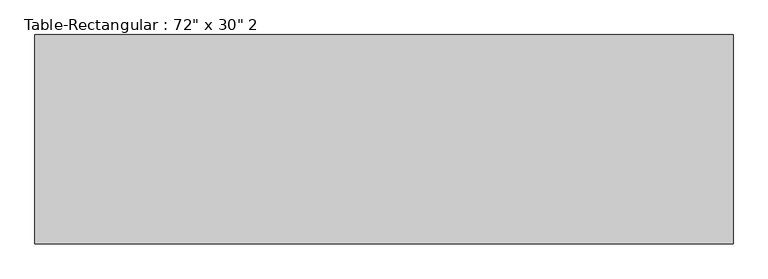
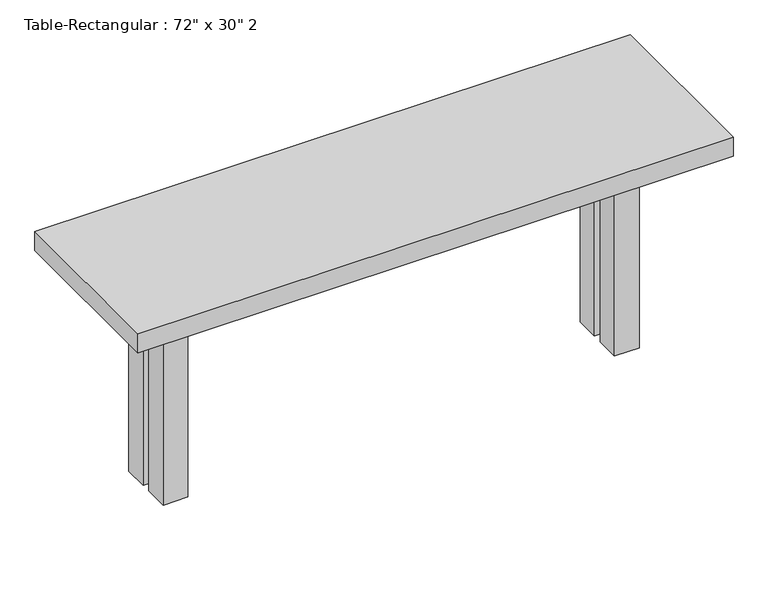
"""IFC4 building model written with IfcOpenShell, lengths in millimetres: furniture geometry."""

from ifc_helpers import new_model, si_unit, frame, origin, origin_with_axes, place, context, project, spatial, polyline, outline, extrude, source, transform, mapped, element, save


def furniture_87306a90(model_context):
    return source(origin(), model_context, "Body", "SweptSolid", [
        extrude(outline(polyline([(546.1, 38.1), (546.1, 12.7), (-546.1, 12.7), (-546.1, 38.1), (546.1, 38.1)])), frame((0.0, 0.0, 457.2), z_axis=(0.0, 0.0, 1.0), x_axis=(1.0, 0.0, 0.0)), (0.0, 0.0, 1.0), 101.6),
        extrude(outline(polyline([(546.1, -38.1), (-546.1, -38.1), (-546.1, -12.7), (546.1, -12.7), (546.1, -38.1)])), frame((0.0, 0.0, 457.2), z_axis=(0.0, 0.0, 1.0), x_axis=(1.0, 0.0, 0.0)), (0.0, 0.0, 1.0), 101.6),
        extrude(outline(polyline([(-558.8, -12.7), (-584.2, -12.7), (-584.2, 12.7), (-558.8, 12.7), (-558.8, -12.7)])), frame((0.0, 0.0, 457.2), z_axis=(0.0, 0.0, 1.0), x_axis=(1.0, 0.0, 0.0)), (0.0, 0.0, 1.0), 101.6),
        extrude(outline(polyline([(558.8, -12.7), (558.8, 12.7), (584.2, 12.7), (584.2, -12.7), (558.8, -12.7)])), frame((0.0, 0.0, 457.2), z_axis=(0.0, 0.0, 1.0), x_axis=(1.0, 0.0, 0.0)), (0.0, 0.0, 1.0), 101.6),
        extrude(outline(polyline([(762.0, 228.6), (762.0, -228.6), (-762.0, -228.6), (-762.0, 228.6), (762.0, 228.6)])), frame((0.0, 0.0, 558.8), z_axis=(0.0, 0.0, 1.0), x_axis=(1.0, 0.0, 0.0)), (0.0, 0.0, 1.0), 50.8),
        extrude(outline(polyline([(-546.1, 76.2), (-546.1, 12.7), (-609.6, 12.7), (-609.6, 76.2), (-546.1, 76.2)])), origin_with_axes(), (0.0, 0.0, 1.0), 558.8),
        extrude(outline(polyline([(546.1, 76.2), (609.6, 76.2), (609.6, 12.7), (546.1, 12.7), (546.1, 76.2)])), origin_with_axes(), (0.0, 0.0, 1.0), 558.8),
        extrude(outline(polyline([(-546.1, -76.2), (-609.6, -76.2), (-609.6, -12.7), (-546.1, -12.7), (-546.1, -76.2)])), origin_with_axes(), (0.0, 0.0, 1.0), 558.8),
        extrude(outline(polyline([(546.1, -76.2), (546.1, -12.7), (609.6, -12.7), (609.6, -76.2), (546.1, -76.2)])), origin_with_axes(), (0.0, 0.0, 1.0), 558.8),
    ])


if __name__ == "__main__":
    model = new_model("IFC4")
    model_context = context("Model", 3, world=origin())
    ifc_project = project(units=[si_unit("LENGTHUNIT", "METRE", prefix="MILLI")], contexts=[model_context])
    site = spatial("IfcSite", under=ifc_project)
    building = spatial("IfcBuilding", under=site)
    placement = place(None, origin())
    furniture_shape = furniture_87306a90(model_context)
    element("IfcFurniture", 1, ObjectType="Table-Rectangular : 72\" x 30\" 2", at=placement, inside=building, context=model_context, shape_type="MappedRepresentation", body=[
        mapped(furniture_shape, transform((0.0, 0.0, 0.0), x_axis=(1.0, 0.0, 0.0), y_axis=(0.0, 1.0, 0.0), z_axis=(0.0, 0.0, 1.0))),
    ])
    save(model, "model.ifc")

# Revit data of these elements
# Type "Table-Rectangular : 72\" x 30\" 2"
#   Assembly Code = "E2020200"
#   Height = 2' - 0"
#   Length = 5' - 0"
#   Width = 1' - 6"
#   Base Material = Birch
#   Top Material = Birch
#   Default Elevation = 0
# Element 1 (IfcFurniture, "Table-Rectangular : 72\" x 30\" 2")
#   Materials on its faces: "Birch"
# Materials
#   "Birch": class "Wood", colour RGB 210 159 95, transparency 0, Description = "Betula Alleghaniensis", Cost = 0
